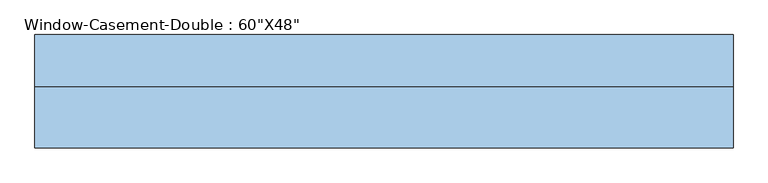
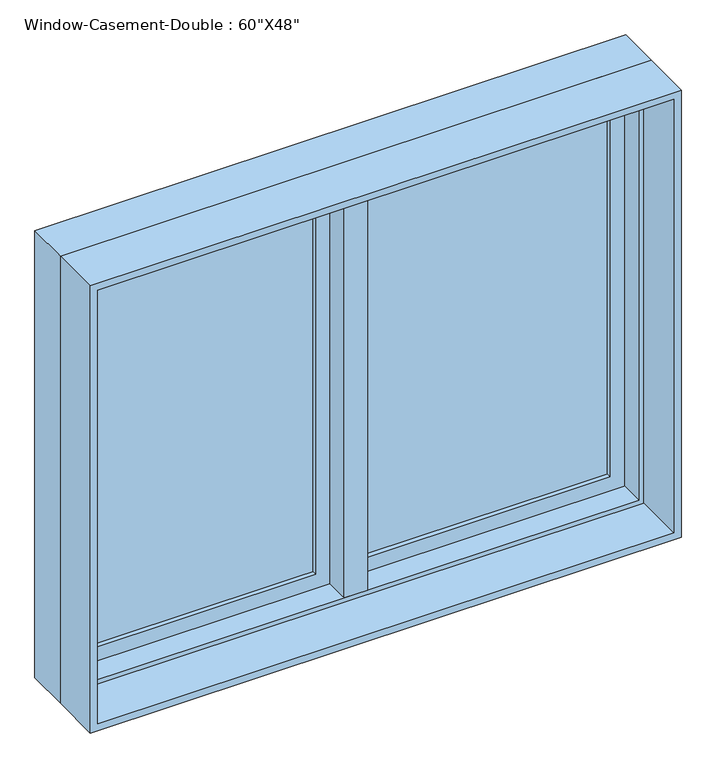
"""IFC4 building model written with IfcOpenShell, lengths in millimetres: window geometry."""

from ifc_helpers import new_model, si_unit, frame, origin, place, context, project, spatial, polyline, outline, extrude, faceted_brep, source, transform, mapped, element, save


def window_178678fa(model_context):
    return source(origin(), model_context, "Body", "SolidModel", [
        faceted_brep([(9.525, 133.35, 2120.9), (-9.525, 133.35, 2120.9), (-9.525, 82.55, 2120.9), (9.525, 82.55, 2120.9), (9.525, 133.35, 927.1), (9.525, 82.55, 927.1), (-9.525, 82.55, 927.1), (-9.525, 133.35, 927.1), (-9.525, 82.55, 946.15), (-9.525, 82.55, 2101.85), (-30.1625, 82.55, 946.15), (-30.1625, 82.55, 2101.85), (-30.1625, 19.05, 946.15), (-30.1625, 19.05, 2101.85), (30.1625, 19.05, 946.15), (30.1625, 19.05, 2101.85), (30.1625, 82.55, 946.15), (30.1625, 82.55, 2101.85), (9.525, 82.55, 946.15), (9.525, 82.55, 2101.85)], [[[0, 1, 2, 3]], [[4, 5, 6, 7]], [[1, 0, 4, 7]], [[2, 1, 7, 6, 8, 9]], [[9, 8, 10, 11]], [[11, 10, 12, 13]], [[13, 12, 14, 15]], [[15, 14, 16, 17]], [[17, 16, 18, 19]], [[0, 3, 19, 18, 5, 4]], [[18, 8, 6, 5]], [[9, 19, 3, 2]], [[8, 18, 16, 14, 12, 10]], [[19, 9, 11, 13, 15, 17]]]),
        extrude(outline(polyline([(-66.675, 114.3), (-66.675, 107.95), (-692.15, 107.95), (-692.15, 114.3), (-66.675, 114.3)])), frame((0.0, 0.0, 984.25), z_axis=(0.0, 0.0, 1.0), x_axis=(1.0, 0.0, 0.0)), (0.0, 0.0, 1.0), 1079.5),
        extrude(outline(polyline([(-692.15, 95.25), (-692.15, 101.6), (-66.675, 101.6), (-66.675, 95.25), (-692.15, 95.25)])), frame((0.0, 0.0, 984.25), z_axis=(0.0, 0.0, 1.0), x_axis=(1.0, 0.0, 0.0)), (0.0, 0.0, 1.0), 1079.5),
        extrude(outline(polyline([(692.15, 114.3), (692.15, 107.95), (66.675, 107.95), (66.675, 114.3), (692.15, 114.3)])), frame((0.0, 0.0, 984.25), z_axis=(0.0, 0.0, 1.0), x_axis=(1.0, 0.0, 0.0)), (0.0, 0.0, 1.0), 1079.5),
        extrude(outline(polyline([(66.675, 95.25), (66.675, 101.6), (692.15, 101.6), (692.15, 95.25), (66.675, 95.25)])), frame((0.0, 0.0, 984.25), z_axis=(0.0, 0.0, 1.0), x_axis=(1.0, 0.0, 0.0)), (0.0, 0.0, 1.0), 1079.5),
        extrude(outline(polyline([(2120.9, -749.3), (927.1, -749.3), (927.1, -9.525), (2120.9, -9.525), (2120.9, -749.3)]), holes=[polyline([(2063.75, -66.675), (984.25, -66.675), (984.25, -692.15), (2063.75, -692.15), (2063.75, -66.675)])]), frame((0.0, 82.55, 0.0), z_axis=(0.0, 1.0, 0.0), x_axis=(0.0, 0.0, 1.0)), (0.0, 0.0, 1.0), 44.45),
        extrude(outline(polyline([(927.1, 749.3), (2120.9, 749.3), (2120.9, 9.525), (927.1, 9.525), (927.1, 749.3)]), holes=[polyline([(984.25, 66.675), (2063.75, 66.675), (2063.75, 692.15), (984.25, 692.15), (984.25, 66.675)])]), frame((0.0, 82.55, 0.0), z_axis=(0.0, 1.0, 0.0), x_axis=(0.0, 0.0, 1.0)), (0.0, 0.0, 1.0), 44.45),
        extrude(outline(polyline([(2133.6, -762.0), (914.4, -762.0), (914.4, 762.0), (2133.6, 762.0), (2133.6, -762.0)]), holes=[polyline([(2114.55, 742.95), (933.45, 742.95), (933.45, -742.95), (2114.55, -742.95), (2114.55, 742.95)])]), frame((0.0, -114.3, 0.0), z_axis=(0.0, 1.0, 0.0), x_axis=(0.0, 0.0, 1.0)), (0.0, 0.0, 1.0), 133.35),
        faceted_brep([(730.25, 82.55, 2101.85), (730.25, 19.05, 2101.85), (-730.25, 19.05, 2101.85), (-730.25, 82.55, 2101.85), (749.3, 133.35, 2120.9), (749.3, 82.55, 2120.9), (-749.3, 82.55, 2120.9), (-749.3, 133.35, 2120.9), (762.0, 19.05, 2133.6), (762.0, 133.35, 2133.6), (-762.0, 133.35, 2133.6), (-762.0, 19.05, 2133.6), (-730.25, 19.05, 946.15), (-730.25, 82.55, 946.15), (-749.3, 82.55, 927.1), (-749.3, 133.35, 927.1), (-762.0, 133.35, 914.4), (-762.0, 19.05, 914.4), (730.25, 19.05, 946.15), (730.25, 82.55, 946.15), (749.3, 82.55, 927.1), (749.3, 133.35, 927.1), (762.0, 133.35, 914.4), (762.0, 19.05, 914.4)], [[[0, 1, 2, 3]], [[4, 5, 6, 7]], [[8, 9, 10, 11]], [[3, 2, 12, 13]], [[7, 6, 14, 15]], [[11, 10, 16, 17]], [[13, 12, 18, 19]], [[15, 14, 20, 21]], [[17, 16, 22, 23]], [[11, 17, 23, 8], [1, 18, 12, 2]], [[19, 18, 1, 0]], [[5, 20, 14, 6], [3, 13, 19, 0]], [[21, 20, 5, 4]], [[23, 22, 9, 8]], [[9, 22, 16, 10], [7, 15, 21, 4]]]),
    ])


if __name__ == "__main__":
    model = new_model("IFC4")
    model_context = context("Model", 3, world=origin())
    ifc_project = project(units=[si_unit("LENGTHUNIT", "METRE", prefix="MILLI")], contexts=[model_context])
    site = spatial("IfcSite", under=ifc_project)
    building = spatial("IfcBuilding", under=site)
    placement = place(None, origin())
    window_shape = window_178678fa(model_context)
    element("IfcWindow", 1, ObjectType="Window-Casement-Double : 60\"X48\"", at=placement, inside=building, context=model_context, shape_type="MappedRepresentation", body=[
        mapped(window_shape, transform((0.0, 0.0, 0.0), x_axis=(1.0, 0.0, 0.0), y_axis=(0.0, 1.0, 0.0), z_axis=(0.0, 0.0, 1.0))),
    ])
    save(model, "model.ifc")

# Revit data of these elements
# Type "Window-Casement-Double : 60\"X48\""
#   Type Mark = "W"
#   Fire Rating = "0.5h"
#   Assembly Code = "B2020100"
#   Analytic Construction = "Double glazing - domestic"
#   Frame Extension [instance default] = 0' - 0 1/4"
#   Window Inset [instance default] = 0' - 0"
#   Wall Thickness [instance default] = 0' - 6"
#   Interior Wall Closure [instance default] = 0' - 2 1/4"
#   Half Width = 2' - 6"
#   Visual Light Transmittance = 0.81
#   Thermal Resistance (R) = 1.8146 (h·ft²·°F)/BTU
#   Solar Heat Gain Coefficient = 0.76
#   Rough Width = 5' - 0 1/2"
#   Rough Height = 4' - 0 1/2"
#   Height = 4' - 0"
#   Heat Transfer Coefficient (U) = 0.5511 BTU/(h·ft²·°F)
#   Exterior Wall Closure [instance default] = 0' - 1 1/4"
#   Extension Jamb [instance default] = 0' - 2 1/4"
#   Default Sill Height = 3' - 0"
#   Width = 5' - 0"
#   Muntin Visibility = yes
#   Interior Trim Visibility [instance default] = yes
#   Exterior Trim Visibility [instance default] = yes
#   Extension Jamb Visibility [instance default] = yes
#   Interior Trim Material = Wood - Stained
#   Muntin Pattern = Muntin Pattern_2x2 : Muntin Pattern_2x2
#   Interior Trim = Trim-Window-Interior-Flat : Picture Frame
#   Interior Frame Material = Wood - Stained
#   Glass Panel Material = Glass
#   Exterior Trim Material = Clad - White
#   Exterior Trim = Trim-Window-Exterior-Flat : with Sill
#   Exterior Frame Material = Clad - White
#   Wall Closure = (empty or 0)
# Element 1 (IfcWindow, "Window-Casement-Double : 60\"X48\"")
#   Wall Thickness = 0' - 9"
#   Extension Jamb = 0' - 5 1/4"
#   Materials on its faces: "Wood - Stained", "Glass", "Clad - White"
# Materials
#   "Wood - Stained": class "Wood", colour RGB 224 178 126, transparency 0, Cost = 0
#   "Glass": class "Glass", colour RGB 0 128 192, transparency 0.75, Description = "Soda Lime Glass", Cost = 0
#   "Clad - White": class "Wood", colour RGB 242 242 238, transparency 0, Cost = 0
